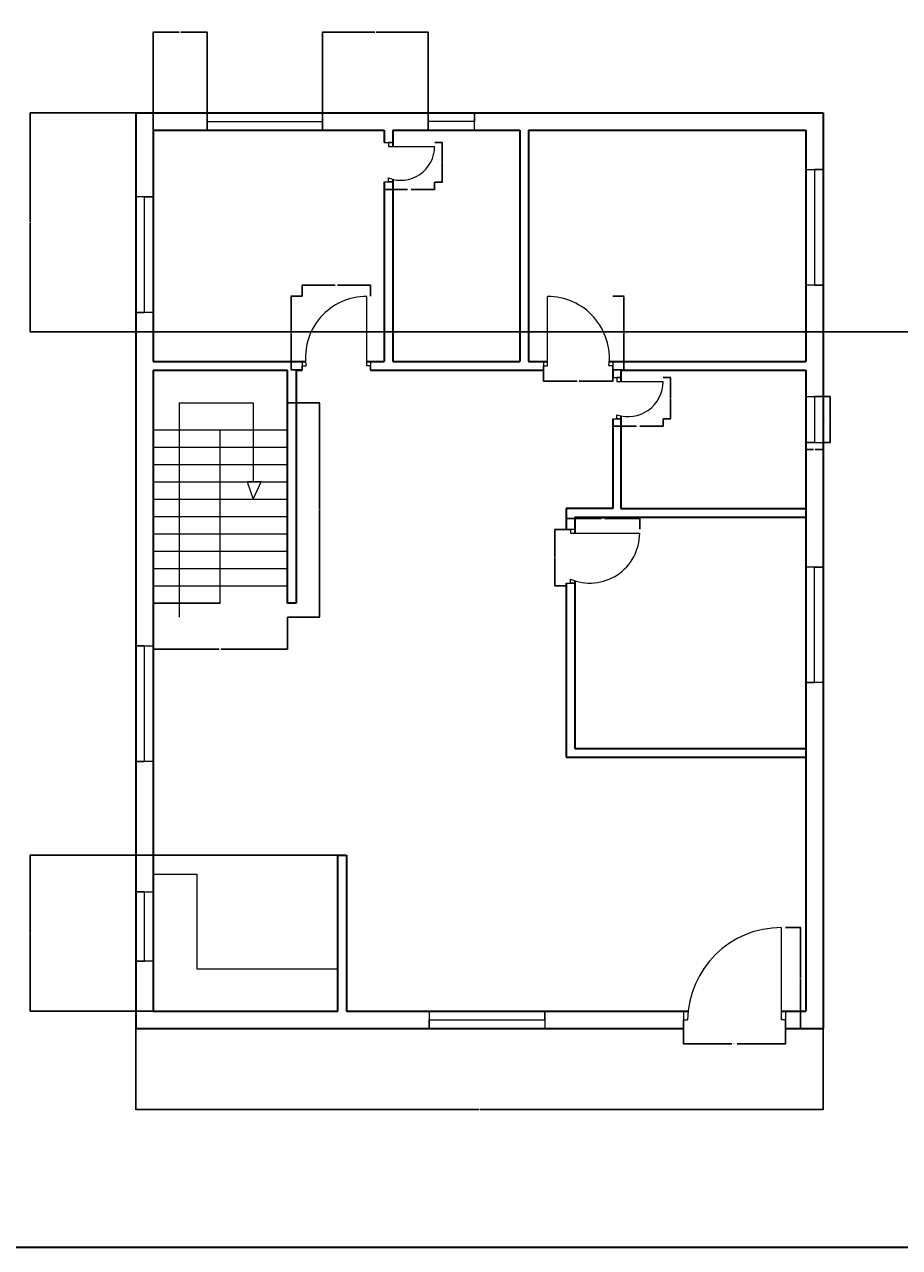
# Model space of a CAD drawing. Units: inches. Extents: x 1912 to 3731, y 1384 to 2459.
# Tile 6 of 8: x 2821 to 3276, y 1384 to 2019. Entities that reach past the tile are written whole.
import ezdxf

# ---------------------------------------------------------------- set-up
doc = ezdxf.new("R2010")
doc.units = ezdxf.units.IN
for name, color, linetype, lineweight in [('A-ANNO-DIMS', 2, 'Continuous', 18), ('A-ANNO-SYMB', 2, 'Continuous', 25), ('A-ANNO-TTLB', 7, 'Continuous', 35), ('A-DOOR', 3, 'Continuous', 20), ('A-FLOR-CASE', 8, 'Continuous', 20), ('A-FLOR-STRS', 7, 'Continuous', 18), ('A-GLAZ', 4, 'Continuous', 18), ('A-WALL', 7, 'Continuous', 35)]:
    doc.layers.add(name, color=color, linetype=linetype, lineweight=lineweight)
doc.styles.get("Standard").update_dxf_attribs({"font": 'arial.ttf'})
doc.dimstyles.get("Standard").update_dxf_attribs({"dimtxt": 0.18, "dimasz": 0.18, "dimexe": 0.18, "dimexo": 0.0625, "dimgap": 0.09, "dimtad": 0, "dimtih": 1, "dimtoh": 1, "dimdec": 4, "dimzin": 0, "dimdsep": 46, "dimtxsty": 'Standard', "dimcen": 0.09, "dimadec": 0, "dimazin": 0, "dimtfac": 1, "dimtdec": 4, "dimtofl": 0, "dimtmove": 0, "dimatfit": 3, "dimfxl": 1, "dimtolj": 1, "dimtzin": 0, "dimarcsym": 0})

# ---------------------------------------------------------------- blocks, each defined once
blk = doc.blocks.new('STAIR-RETURN-GROUND')
for p, q in [((13.73, 0), (13.73, 111.26)), ((13.73, 111.26), (52.04, 111.26)), ((52.04, 111.26), (52.04, 70.24)), ((0, 97.24), (34.87, 97.24)), ((34.87, 97.24), (69.75, 97.24)), ((34.87, 7.24), (34.87, 97.12)), ((0, 88.24), (34.87, 88.24)), ((34.87, 88.24), (69.75, 88.24)), ((0, 79.24), (34.87, 79.24)), ((34.87, 79.24), (69.75, 79.24)), ((0, 70.24), (34.87, 70.24)), ((34.87, 70.24), (69.75, 70.24)), ((56.12, 70.24), (48.82, 70.24)), ((48.82, 70.24), (52.04, 61.24)), ((52.04, 61.24), (56.12, 70.24)), ((0, 61.24), (34.87, 61.24)), ((34.87, 61.24), (69.75, 61.24)), ((0, 52.24), (34.87, 52.24)), ((34.87, 52.24), (69.75, 52.24)), ((0, 43.24), (34.87, 43.24)), ((34.87, 43.24), (69.75, 43.24)), ((0, 34.24), (34.87, 34.24)), ((34.87, 34.24), (69.75, 34.24)), ((0, 25.24), (34.87, 25.24)), ((34.87, 25.24), (69.75, 25.24)), ((0, 16.24), (34.87, 16.24)), ((34.87, 7.24), (34.87, 16.24)), ((34.87, 16.24), (69.75, 16.24)), ((34.87, 7.24), (0, 7.24)), ((0, 7.24), (34.87, 7.24))]:
    blk.add_line(p, q)
blk = doc.blocks.new('DOOR-36-GF-KIDS')
for p, q in [((2, 2.25), (2, 38.25)), ((0, 4.5), (0, 0)), ((0, 0), (0, 2.25)), ((0, 2.25), (2, 2.25)), ((35.93, 2.25), (33.93, 2.25)), ((35.93, 4.5), (35.93, 0)), ((35.93, 0), (35.93, 2.25))]:
    blk.add_line(p, q)
blk.add_arc((2, 6.09), 32.16, 353.14548, 90)
blk = doc.blocks.new('DOOR-36-GF-MASTER')
for p, q in [((33.51, 2.25), (33.51, 38.25)), ((0, 4.5), (0, 0)), ((0, 0), (0, 2.25)), ((0, 2.25), (2, 2.25)), ((35.51, 2.25), (33.51, 2.25)), ((35.51, 4.5), (35.51, 0)), ((35.51, 0), (35.51, 2.25))]:
    blk.add_line(p, q)
blk.add_arc((33.51, 6.46), 31.79, 90, 187.60289)
blk = doc.blocks.new('DOOR-24-GF-ENSUITE')
for p, q in [((0, 20.44), (4.5, 20.44)), ((4.5, 20.44), (2.25, 20.44)), ((2.25, 20.44), (2.25, 18.44)), ((2.25, 18.44), (26.25, 18.44)), ((2.25, 0), (2.25, 2)), ((0, 0), (4.5, 0)), ((4.5, 0), (2.25, 0))]:
    blk.add_line(p, q)
blk.add_arc((8.62, 18.44), 17.63, 248.8218, 0)
blk = doc.blocks.new('DOOR-24-GF-BATH')
for p, q in [((0, 21.32), (4.21, 21.32)), ((4.21, 21.32), (2.1, 21.32)), ((2.1, 21.32), (2.1, 19.32)), ((2.1, 19.32), (26.1, 19.32)), ((2.1, 0), (2.1, 2)), ((0, 0), (4.21, 0)), ((4.21, 0), (2.1, 0))]:
    blk.add_line(p, q)
blk.add_arc((7.86, 19.32), 18.25, 251.63069, 0)
blk = doc.blocks.new('DOOR-36-GF-FAMILY')
for p, q in [((4.5, 27.89), (0, 27.89)), ((0, 27.89), (2.25, 27.89)), ((2.25, 27.89), (2.25, 25.89)), ((2.25, 25.89), (38.25, 25.89)), ((0, 0.04), (4.5, 0.04)), ((2.25, 0.04), (2.25, 2.04)), ((4.5, 0.04), (2.25, 0.04))]:
    blk.add_line(p, q)
blk.add_arc((12.35, 25.89), 25.9, 247.04952, 0)
blk = doc.blocks.new('DOOR-48-ENTRY')
for p, q in [((50.83, 40.5), (50.83, 52.5)), ((50.83, 4.5), (50.83, 40.5)), ((0, 9), (0, 0)), ((52.83, 9), (52.83, 0)), ((0, 0), (0, 4.5)), ((0, 4.5), (2, 4.5)), ((52.83, 4.5), (50.83, 4.5)), ((52.83, 0), (52.83, 4.5))]:
    blk.add_line(p, q)
blk.add_arc((50.83, 3.66), 48.84, 90, 179.01371)
blk = doc.blocks.new('WIN-PLAN-60-A')
for p, q in [((0, 9), (0, 0)), ((60, 4.5), (60, 9)), ((60, 9), (60, 0)), ((0, 0), (0, 4.5)), ((0, 4.5), (60, 4.5))]:
    blk.add_line(p, q)
blk = doc.blocks.new('WIN-PLAN-60-B')
for p, q in [((0, 60), (9, 60)), ((9, 60), (4.5, 60)), ((4.5, 60), (4.5, 0)), ((9, 0), (0, 0)), ((4.5, 0), (9, 0))]:
    blk.add_line(p, q)
blk = doc.blocks.new('WIN-PLAN-24-A')
for p, q in [((0, 24), (9, 24)), ((9, 24), (4.5, 24)), ((4.5, 24), (4.5, 0)), ((4.5, 0), (0, 0)), ((0, 0), (9, 0))]:
    blk.add_line(p, q)
blk = doc.blocks.new('WIN-PLAN-36')
for p, q in [((4.5, 36), (0, 36)), ((0, 36), (9, 36)), ((4.5, 0), (4.5, 36)), ((9, 0), (0, 0)), ((0, 0), (4.5, 0))]:
    blk.add_line(p, q)
blk = doc.blocks.new('*D35')
at = {"layer": 'A-ANNO-DIMS', "color": 0, "lineweight": -2, "transparency": 16777216}
for p, q in [((3235.85, 1825.91), (3239.57, 1825.91)), ((3239.39, 1825.73), (3239.39, 1814.1)), ((3239.39, 1802.09), (3239.39, 1813.73)), ((3235.85, 1801.91), (3239.57, 1801.91))]:
    blk.add_line(p, q, dxfattribs=at)
at = {"layer": 'A-ANNO-DIMS', "color": 0, "transparency": 16777216}
for points in [[(3239.36, 1825.73), (3239.42, 1825.73), (3239.39, 1825.91)], [(3239.36, 1802.09), (3239.42, 1802.09), (3239.39, 1801.91)]]:
    blk.add_solid(points, dxfattribs=at)
at = {"layer": 'Defpoints', "color": 0, "transparency": 16777216}
for p in [(3235.79, 1825.91), (3239.39, 1825.91), (3235.79, 1801.91)]:
    blk.add_point(p, dxfattribs=at)
at = {"layer": 'A-ANNO-DIMS', "color": 0, "transparency": 16777216, "insert": (3239.39, 1813.91), "char_height": 0.18, "attachment_point": 5}
blk.add_mtext('\\A1;WC WINDOW 24 TYP.', dxfattribs=at)
blk = doc.blocks.new('*D36')
at = {"layer": 'A-ANNO-DIMS', "color": 0, "lineweight": -2, "transparency": 16777216}
for p, q in [((3226.79, 1801.85), (3226.79, 1798.13)), ((3226.97, 1798.31), (3230.83, 1798.31)), ((3235.61, 1798.31), (3231.74, 1798.31)), ((3235.79, 1801.85), (3235.79, 1798.13))]:
    blk.add_line(p, q, dxfattribs=at)
at = {"layer": 'A-ANNO-DIMS', "color": 0, "transparency": 16777216}
for points in [[(3226.97, 1798.34), (3226.97, 1798.28), (3226.79, 1798.31)], [(3235.61, 1798.34), (3235.61, 1798.28), (3235.79, 1798.31)]]:
    blk.add_solid(points, dxfattribs=at)
at = {"layer": 'Defpoints', "color": 0, "transparency": 16777216}
for p in [(3226.79, 1801.91), (3235.79, 1801.91), (3235.79, 1798.31)]:
    blk.add_point(p, dxfattribs=at)
at = {"layer": 'A-ANNO-DIMS', "color": 0, "transparency": 16777216, "insert": (3231.29, 1798.31), "char_height": 0.18, "attachment_point": 5}
blk.add_mtext('\\A1;9 TYP.', dxfattribs=at)
blk = doc.blocks.new('*D63')
at = {"layer": 'A-ANNO-DIMS', "color": 0, "lineweight": -2, "transparency": 16777216}
for p, q in [((2957.59, 1822.61), (2974.4, 1822.61)), ((2974.22, 1822.43), (2974.22, 1767.16)), ((2974.22, 1711.53), (2974.22, 1766.79)), ((2957.59, 1711.35), (2974.4, 1711.35))]:
    blk.add_line(p, q, dxfattribs=at)
at = {"layer": 'A-ANNO-DIMS', "color": 0, "transparency": 16777216}
for points in [[(2974.19, 1822.43), (2974.25, 1822.43), (2974.22, 1822.61)], [(2974.19, 1711.53), (2974.25, 1711.53), (2974.22, 1711.35)]]:
    blk.add_solid(points, dxfattribs=at)
at = {"layer": 'Defpoints', "color": 0, "transparency": 16777216}
for p in [(2957.53, 1822.61), (2974.22, 1822.61), (2957.53, 1711.35)]:
    blk.add_point(p, dxfattribs=at)
at = {"layer": 'A-ANNO-DIMS', "color": 0, "transparency": 16777216, "insert": (2974.22, 1766.98), "char_height": 0.18, "attachment_point": 5}
blk.add_mtext('\\A1;STAIR 111 TYP.', dxfattribs=at)
blk = doc.blocks.new('*D64')
at = {"layer": 'A-ANNO-DIMS', "color": 0, "lineweight": -2, "transparency": 16777216}
for p, q in [((2887.79, 1711.28), (2887.79, 1694.48)), ((2957.53, 1711.28), (2957.53, 1694.48)), ((2887.97, 1694.66), (2922.13, 1694.66)), ((2957.35, 1694.66), (2923.19, 1694.66))]:
    blk.add_line(p, q, dxfattribs=at)
at = {"layer": 'A-ANNO-DIMS', "color": 0, "transparency": 16777216}
for points in [[(2887.97, 1694.69), (2887.97, 1694.63), (2887.79, 1694.66)], [(2957.35, 1694.69), (2957.35, 1694.63), (2957.53, 1694.66)]]:
    blk.add_solid(points, dxfattribs=at)
at = {"layer": 'Defpoints', "color": 0, "transparency": 16777216}
for p in [(2887.79, 1711.35), (2957.53, 1711.35), (2957.53, 1694.66)]:
    blk.add_point(p, dxfattribs=at)
at = {"layer": 'A-ANNO-DIMS', "color": 0, "transparency": 16777216, "insert": (2922.66, 1694.66), "char_height": 0.18, "attachment_point": 5}
blk.add_mtext('\\A1;70 TYP.', dxfattribs=at)
blk = doc.blocks.new('*D67')
at = {"layer": 'A-ANNO-DIMS', "color": 0, "lineweight": -2, "transparency": 16777216}
for p, q in [((3126.64, 1877.88), (3132.49, 1877.88)), ((3132.31, 1877.7), (3132.31, 1858.93)), ((3132.31, 1839.81), (3132.31, 1858.57)), ((3126.64, 1839.63), (3132.49, 1839.63))]:
    blk.add_line(p, q, dxfattribs=at)
at = {"layer": 'A-ANNO-DIMS', "color": 0, "transparency": 16777216}
for points in [[(3132.28, 1877.7), (3132.34, 1877.7), (3132.31, 1877.88)], [(3132.28, 1839.81), (3132.34, 1839.81), (3132.31, 1839.63)]]:
    blk.add_solid(points, dxfattribs=at)
at = {"layer": 'Defpoints', "color": 0, "transparency": 16777216}
for p in [(3126.58, 1877.88), (3132.31, 1877.88), (3126.58, 1839.63)]:
    blk.add_point(p, dxfattribs=at)
at = {"layer": 'A-ANNO-DIMS', "color": 0, "transparency": 16777216, "insert": (3132.31, 1858.75), "char_height": 0.18, "attachment_point": 5}
blk.add_mtext('\\A1;DOOR 38 TYP.', dxfattribs=at)
blk = doc.blocks.new('*D68')
at = {"layer": 'A-ANNO-DIMS', "color": 0, "lineweight": -2, "transparency": 16777216}
for p, q in [((3090.64, 1839.56), (3090.64, 1833.71)), ((3126.58, 1839.56), (3126.58, 1833.71)), ((3090.82, 1833.89), (3108.08, 1833.89)), ((3126.4, 1833.89), (3109.14, 1833.89))]:
    blk.add_line(p, q, dxfattribs=at)
at = {"layer": 'A-ANNO-DIMS', "color": 0, "transparency": 16777216}
for points in [[(3090.82, 1833.92), (3090.82, 1833.86), (3090.64, 1833.89)], [(3126.4, 1833.92), (3126.4, 1833.86), (3126.58, 1833.89)]]:
    blk.add_solid(points, dxfattribs=at)
at = {"layer": 'Defpoints', "color": 0, "transparency": 16777216}
for p in [(3090.64, 1839.63), (3126.58, 1839.63), (3126.58, 1833.89)]:
    blk.add_point(p, dxfattribs=at)
at = {"layer": 'A-ANNO-DIMS', "color": 0, "transparency": 16777216, "insert": (3108.61, 1833.89), "char_height": 0.18, "attachment_point": 5}
blk.add_mtext('\\A1;36 TYP.', dxfattribs=at)
blk = doc.blocks.new('*D69')
at = {"layer": 'A-ANNO-DIMS', "color": 0, "lineweight": -2, "transparency": 16777216}
for p, q in [((2965.17, 1877.88), (2959.31, 1877.88)), ((2959.49, 1877.7), (2959.49, 1858.93)), ((2959.49, 1839.81), (2959.49, 1858.57)), ((2965.17, 1839.63), (2959.31, 1839.63))]:
    blk.add_line(p, q, dxfattribs=at)
at = {"layer": 'A-ANNO-DIMS', "color": 0, "transparency": 16777216}
for points in [[(2959.46, 1877.7), (2959.52, 1877.7), (2959.49, 1877.88)], [(2959.46, 1839.81), (2959.52, 1839.81), (2959.49, 1839.63)]]:
    blk.add_solid(points, dxfattribs=at)
at = {"layer": 'Defpoints', "color": 0, "transparency": 16777216}
for p in [(2959.49, 1877.88), (2965.23, 1877.88), (2965.23, 1839.63)]:
    blk.add_point(p, dxfattribs=at)
at = {"layer": 'A-ANNO-DIMS', "color": 0, "transparency": 16777216, "insert": (2959.49, 1858.75), "char_height": 0.18, "attachment_point": 5}
blk.add_mtext('\\A1;DOOR 38 TYP.', dxfattribs=at)
blk = doc.blocks.new('*D70')
at = {"layer": 'A-ANNO-DIMS', "color": 0, "lineweight": -2, "transparency": 16777216}
for p, q in [((2965.23, 1877.94), (2965.23, 1883.79)), ((2965.41, 1883.61), (2982.46, 1883.61)), ((3000.56, 1883.61), (2983.51, 1883.61)), ((3000.74, 1877.94), (3000.74, 1883.79))]:
    blk.add_line(p, q, dxfattribs=at)
at = {"layer": 'A-ANNO-DIMS', "color": 0, "transparency": 16777216}
for points in [[(2965.41, 1883.64), (2965.41, 1883.58), (2965.23, 1883.61)], [(3000.56, 1883.64), (3000.56, 1883.58), (3000.74, 1883.61)]]:
    blk.add_solid(points, dxfattribs=at)
at = {"layer": 'Defpoints', "color": 0, "transparency": 16777216}
for p in [(3000.74, 1883.61), (2965.23, 1877.88), (3000.74, 1877.88)]:
    blk.add_point(p, dxfattribs=at)
at = {"layer": 'A-ANNO-DIMS', "color": 0, "transparency": 16777216, "insert": (2982.99, 1883.61), "char_height": 0.18, "attachment_point": 5}
blk.add_mtext('\\A1;36 TYP.', dxfattribs=at)
blk = doc.blocks.new('*D71')
at = {"layer": 'A-ANNO-DIMS', "color": 0, "lineweight": -2, "transparency": 16777216}
for p, q in [((3007.79, 1937.16), (3007.79, 1933.11)), ((3034.04, 1937.16), (3034.04, 1933.11)), ((3007.97, 1933.29), (3019.97, 1933.29)), ((3033.86, 1933.29), (3021.85, 1933.29))]:
    blk.add_line(p, q, dxfattribs=at)
at = {"layer": 'A-ANNO-DIMS', "color": 0, "transparency": 16777216}
for points in [[(3007.97, 1933.32), (3007.97, 1933.26), (3007.79, 1933.29)], [(3033.86, 1933.32), (3033.86, 1933.26), (3034.04, 1933.29)]]:
    blk.add_solid(points, dxfattribs=at)
at = {"layer": 'Defpoints', "color": 0, "transparency": 16777216}
for p in [(3007.79, 1937.22), (3034.04, 1937.22), (3034.04, 1933.29)]:
    blk.add_point(p, dxfattribs=at)
at = {"layer": 'A-ANNO-DIMS', "color": 0, "transparency": 16777216, "insert": (3020.91, 1933.29), "char_height": 0.18, "attachment_point": 5}
blk.add_mtext('\\A1;DOOR 26 TYP.', dxfattribs=at)
blk = doc.blocks.new('*D72')
at = {"layer": 'A-ANNO-DIMS', "color": 0, "lineweight": -2, "transparency": 16777216}
for p, q in [((3034.1, 1957.76), (3038.15, 1957.76)), ((3037.97, 1957.58), (3037.97, 1947.67)), ((3037.97, 1937.4), (3037.97, 1947.31)), ((3034.1, 1937.22), (3038.15, 1937.22))]:
    blk.add_line(p, q, dxfattribs=at)
at = {"layer": 'A-ANNO-DIMS', "color": 0, "transparency": 16777216}
for points in [[(3037.94, 1957.58), (3038, 1957.58), (3037.97, 1957.76)], [(3037.94, 1937.4), (3038, 1937.4), (3037.97, 1937.22)]]:
    blk.add_solid(points, dxfattribs=at)
at = {"layer": 'Defpoints', "color": 0, "transparency": 16777216}
for p in [(3034.04, 1957.76), (3037.97, 1957.76), (3034.04, 1937.22)]:
    blk.add_point(p, dxfattribs=at)
at = {"layer": 'A-ANNO-DIMS', "color": 0, "transparency": 16777216, "insert": (3037.97, 1947.49), "char_height": 0.18, "attachment_point": 5}
blk.add_mtext('\\A1;21 TYP.', dxfattribs=at)
blk = doc.blocks.new('*D73')
at = {"layer": 'A-ANNO-DIMS', "color": 0, "lineweight": -2, "transparency": 16777216}
for p, q in [((3126.58, 1814.27), (3126.58, 1810.23)), ((3126.76, 1810.41), (3138.69, 1810.41)), ((3152.5, 1810.41), (3140.56, 1810.41)), ((3152.68, 1814.27), (3152.68, 1810.23))]:
    blk.add_line(p, q, dxfattribs=at)
at = {"layer": 'A-ANNO-DIMS', "color": 0, "transparency": 16777216}
for points in [[(3126.76, 1810.44), (3126.76, 1810.38), (3126.58, 1810.41)], [(3152.5, 1810.44), (3152.5, 1810.38), (3152.68, 1810.41)]]:
    blk.add_solid(points, dxfattribs=at)
at = {"layer": 'Defpoints', "color": 0, "transparency": 16777216}
for p in [(3126.58, 1814.33), (3152.68, 1814.33), (3152.68, 1810.41)]:
    blk.add_point(p, dxfattribs=at)
at = {"layer": 'A-ANNO-DIMS', "color": 0, "transparency": 16777216, "insert": (3139.63, 1810.41), "char_height": 0.18, "attachment_point": 5}
blk.add_mtext('\\A1;DOOR 26 TYP.', dxfattribs=at)
blk = doc.blocks.new('*D74')
at = {"layer": 'A-ANNO-DIMS', "color": 0, "lineweight": -2, "transparency": 16777216}
for p, q in [((3152.74, 1835.65), (3156.78, 1835.65)), ((3156.6, 1835.47), (3156.6, 1825.17)), ((3156.6, 1814.51), (3156.6, 1824.81)), ((3152.74, 1814.33), (3156.78, 1814.33))]:
    blk.add_line(p, q, dxfattribs=at)
at = {"layer": 'A-ANNO-DIMS', "color": 0, "transparency": 16777216}
for points in [[(3156.57, 1835.47), (3156.63, 1835.47), (3156.6, 1835.65)], [(3156.57, 1814.51), (3156.63, 1814.51), (3156.6, 1814.33)]]:
    blk.add_solid(points, dxfattribs=at)
at = {"layer": 'Defpoints', "color": 0, "transparency": 16777216}
for p in [(3152.68, 1835.65), (3156.6, 1835.65), (3152.68, 1814.33)]:
    blk.add_point(p, dxfattribs=at)
at = {"layer": 'A-ANNO-DIMS', "color": 0, "transparency": 16777216, "insert": (3156.6, 1824.99), "char_height": 0.18, "attachment_point": 5}
blk.add_mtext('\\A1;21 TYP.', dxfattribs=at)
blk = doc.blocks.new('*D75')
at = {"layer": 'A-ANNO-DIMS', "color": 0, "lineweight": -2, "transparency": 16777216}
for p, q in [((3102.29, 1756.92), (3102.29, 1762.78)), ((3102.47, 1762.6), (3120.47, 1762.6)), ((3140.36, 1762.6), (3122.35, 1762.6)), ((3140.54, 1756.92), (3140.54, 1762.78))]:
    blk.add_line(p, q, dxfattribs=at)
at = {"layer": 'A-ANNO-DIMS', "color": 0, "transparency": 16777216}
for points in [[(3102.47, 1762.63), (3102.47, 1762.57), (3102.29, 1762.6)], [(3140.36, 1762.63), (3140.36, 1762.57), (3140.54, 1762.6)]]:
    blk.add_solid(points, dxfattribs=at)
at = {"layer": 'Defpoints', "color": 0, "transparency": 16777216}
for p in [(3140.54, 1762.6), (3102.29, 1756.86), (3140.54, 1756.86)]:
    blk.add_point(p, dxfattribs=at)
at = {"layer": 'A-ANNO-DIMS', "color": 0, "transparency": 16777216, "insert": (3121.41, 1762.6), "char_height": 0.18, "attachment_point": 5}
blk.add_mtext('\\A1;DOOR 38 TYP.', dxfattribs=at)
blk = doc.blocks.new('*D76')
at = {"layer": 'A-ANNO-DIMS', "color": 0, "lineweight": -2, "transparency": 16777216}
for p, q in [((3102.22, 1756.86), (3096.37, 1756.86)), ((3096.55, 1756.68), (3096.55, 1742.42)), ((3096.55, 1727.8), (3096.55, 1742.06)), ((3102.22, 1727.62), (3096.37, 1727.62))]:
    blk.add_line(p, q, dxfattribs=at)
at = {"layer": 'A-ANNO-DIMS', "color": 0, "transparency": 16777216}
for points in [[(3096.52, 1756.68), (3096.58, 1756.68), (3096.55, 1756.86)], [(3096.52, 1727.8), (3096.58, 1727.8), (3096.55, 1727.62)]]:
    blk.add_solid(points, dxfattribs=at)
at = {"layer": 'Defpoints', "color": 0, "transparency": 16777216}
for p in [(3096.55, 1756.86), (3102.29, 1756.86), (3102.29, 1727.62)]:
    blk.add_point(p, dxfattribs=at)
at = {"layer": 'A-ANNO-DIMS', "color": 0, "transparency": 16777216, "insert": (3096.55, 1742.24), "char_height": 0.18, "attachment_point": 5}
blk.add_mtext('\\A1;29 TYP.', dxfattribs=at)
blk = doc.blocks.new('*D77')
at = {"layer": 'A-ANNO-DIMS', "color": 0, "lineweight": -2, "transparency": 16777216}
for p, q in [((3163.37, 1497.56), (3163.37, 1489.52)), ((3216.21, 1497.56), (3216.21, 1489.52)), ((3163.55, 1489.7), (3188.39, 1489.7)), ((3216.03, 1489.7), (3191.19, 1489.7))]:
    blk.add_line(p, q, dxfattribs=at)
at = {"layer": 'A-ANNO-DIMS', "color": 0, "transparency": 16777216}
for points in [[(3163.55, 1489.73), (3163.55, 1489.67), (3163.37, 1489.7)], [(3216.03, 1489.73), (3216.03, 1489.67), (3216.21, 1489.7)]]:
    blk.add_solid(points, dxfattribs=at)
at = {"layer": 'Defpoints', "color": 0, "transparency": 16777216}
for p in [(3163.37, 1497.63), (3216.21, 1497.63), (3216.21, 1489.7)]:
    blk.add_point(p, dxfattribs=at)
at = {"layer": 'A-ANNO-DIMS', "color": 0, "transparency": 16777216, "insert": (3189.79, 1489.7), "char_height": 0.18, "attachment_point": 5}
blk.add_mtext('\\A1;ENTRY DOOR 53 TYP.', dxfattribs=at)
blk = doc.blocks.new('*D78')
at = {"layer": 'A-ANNO-DIMS', "color": 0, "lineweight": -2, "transparency": 16777216}
for p, q in [((3216.27, 1550.13), (3224.31, 1550.13)), ((3224.13, 1549.95), (3224.13, 1524.06)), ((3224.13, 1497.81), (3224.13, 1523.69)), ((3216.27, 1497.63), (3224.31, 1497.63))]:
    blk.add_line(p, q, dxfattribs=at)
at = {"layer": 'A-ANNO-DIMS', "color": 0, "transparency": 16777216}
for points in [[(3224.1, 1549.95), (3224.16, 1549.95), (3224.13, 1550.13)], [(3224.1, 1497.81), (3224.16, 1497.81), (3224.13, 1497.63)]]:
    blk.add_solid(points, dxfattribs=at)
at = {"layer": 'Defpoints', "color": 0, "transparency": 16777216}
for p in [(3216.21, 1550.13), (3224.13, 1550.13), (3216.21, 1497.63)]:
    blk.add_point(p, dxfattribs=at)
at = {"layer": 'A-ANNO-DIMS', "color": 0, "transparency": 16777216, "insert": (3224.13, 1523.88), "char_height": 0.18, "attachment_point": 5}
blk.add_mtext('\\A1;53 TYP.', dxfattribs=at)
blk = doc.blocks.new('*D105')
at = {"layer": 'A-ANNO-DIMS', "color": 0, "lineweight": -2, "transparency": 16777216}
for p, q in [((2878.79, 1497.56), (2878.79, 1455.5)), ((3235.79, 1497.56), (3235.79, 1455.5)), ((2878.97, 1455.68), (3057, 1455.68)), ((3235.61, 1455.68), (3057.57, 1455.68))]:
    blk.add_line(p, q, dxfattribs=at)
at = {"layer": 'A-ANNO-DIMS', "color": 0, "transparency": 16777216}
for points in [[(2878.97, 1455.71), (2878.97, 1455.65), (2878.79, 1455.68)], [(3235.61, 1455.71), (3235.61, 1455.65), (3235.79, 1455.68)]]:
    blk.add_solid(points, dxfattribs=at)
at = {"layer": 'Defpoints', "color": 0, "transparency": 16777216}
for p in [(2878.79, 1497.63), (3235.79, 1497.63), (3235.79, 1455.68)]:
    blk.add_point(p, dxfattribs=at)
at = {"layer": 'A-ANNO-DIMS', "color": 0, "transparency": 16777216, "insert": (3057.29, 1455.68), "char_height": 0.18, "attachment_point": 5}
blk.add_mtext('\\A1;357', dxfattribs=at)
blk = doc.blocks.new('*D108')
at = {"layer": 'A-ANNO-DIMS', "color": 0, "lineweight": -2, "transparency": 16777216}
for p, q in [((2878.72, 1973.13), (2823.71, 1973.13)), ((2823.89, 1972.95), (2823.89, 1916.48)), ((2823.89, 1859.65), (2823.89, 1916.11)), ((2865.78, 1859.47), (2823.71, 1859.47))]:
    blk.add_line(p, q, dxfattribs=at)
at = {"layer": 'A-ANNO-DIMS', "color": 0, "transparency": 16777216}
for points in [[(2823.86, 1972.95), (2823.92, 1972.95), (2823.89, 1973.13)], [(2823.86, 1859.65), (2823.92, 1859.65), (2823.89, 1859.47)]]:
    blk.add_solid(points, dxfattribs=at)
at = {"layer": 'Defpoints', "color": 0, "transparency": 16777216}
for p in [(2878.79, 1973.13), (2823.89, 1859.47), (2865.84, 1859.47)]:
    blk.add_point(p, dxfattribs=at)
at = {"layer": 'A-ANNO-DIMS', "color": 0, "transparency": 16777216, "insert": (2823.89, 1916.3), "char_height": 0.18, "attachment_point": 5}
blk.add_mtext('\\A1;113.66', dxfattribs=at)
blk = doc.blocks.new('*D109')
at = {"layer": 'A-ANNO-DIMS', "color": 0, "lineweight": -2, "transparency": 16777216}
for p, q in [((2887.79, 1964.19), (2887.79, 2015.26)), ((2887.97, 2015.08), (2901.41, 2015.08)), ((2915.64, 2015.08), (2902.2, 2015.08)), ((2915.82, 1964.19), (2915.82, 2015.26))]:
    blk.add_line(p, q, dxfattribs=at)
at = {"layer": 'A-ANNO-DIMS', "color": 0, "transparency": 16777216}
for points in [[(2887.97, 2015.11), (2887.97, 2015.05), (2887.79, 2015.08)], [(2915.64, 2015.11), (2915.64, 2015.05), (2915.82, 2015.08)]]:
    blk.add_solid(points, dxfattribs=at)
at = {"layer": 'Defpoints', "color": 0, "transparency": 16777216}
for p in [(2915.82, 2015.08), (2887.79, 1964.13), (2915.82, 1964.13)]:
    blk.add_point(p, dxfattribs=at)
at = {"layer": 'A-ANNO-DIMS', "color": 0, "transparency": 16777216, "insert": (2901.8, 2015.08), "char_height": 0.18, "attachment_point": 5}
blk.add_mtext('\\A1;28.03', dxfattribs=at)
blk = doc.blocks.new('*D110')
at = {"layer": 'A-ANNO-DIMS', "color": 0, "lineweight": -2, "transparency": 16777216}
for p, q in [((2975.82, 1964.19), (2975.82, 2015.26)), ((2976, 2015.08), (3002.89, 2015.08)), ((3030.56, 2015.08), (3003.67, 2015.08)), ((3030.74, 1964.19), (3030.74, 2015.26))]:
    blk.add_line(p, q, dxfattribs=at)
at = {"layer": 'A-ANNO-DIMS', "color": 0, "transparency": 16777216}
for points in [[(2976, 2015.11), (2976, 2015.05), (2975.82, 2015.08)], [(3030.56, 2015.11), (3030.56, 2015.05), (3030.74, 2015.08)]]:
    blk.add_solid(points, dxfattribs=at)
at = {"layer": 'Defpoints', "color": 0, "transparency": 16777216}
for p in [(3030.74, 2015.08), (2975.82, 1964.13), (3030.74, 1964.13)]:
    blk.add_point(p, dxfattribs=at)
at = {"layer": 'A-ANNO-DIMS', "color": 0, "transparency": 16777216, "insert": (3003.28, 2015.08), "char_height": 0.18, "attachment_point": 5}
blk.add_mtext('\\A1;54.92', dxfattribs=at)
blk = doc.blocks.new('*D111')
at = {"layer": 'A-ANNO-DIMS', "color": 0, "lineweight": -2, "transparency": 16777216}
for p, q in [((2983.72, 1587.72), (2823.71, 1587.72)), ((2823.89, 1587.54), (2823.89, 1547.35)), ((2823.89, 1506.81), (2823.89, 1546.99)), ((2983.72, 1506.63), (2823.71, 1506.63))]:
    blk.add_line(p, q, dxfattribs=at)
at = {"layer": 'A-ANNO-DIMS', "color": 0, "transparency": 16777216}
for points in [[(2823.86, 1587.54), (2823.92, 1587.54), (2823.89, 1587.72)], [(2823.86, 1506.81), (2823.92, 1506.81), (2823.89, 1506.63)]]:
    blk.add_solid(points, dxfattribs=at)
at = {"layer": 'Defpoints', "color": 0, "transparency": 16777216}
for p in [(2823.89, 1587.72), (2983.79, 1587.72), (2983.79, 1506.63)]:
    blk.add_point(p, dxfattribs=at)
at = {"layer": 'A-ANNO-DIMS', "color": 0, "transparency": 16777216, "insert": (2823.89, 1547.17), "char_height": 0.18, "attachment_point": 5}
blk.add_mtext('\\A1;81.09', dxfattribs=at)

msp = doc.modelspace()

# ---------------------------------------------------------------- linework, layer by layer
at = {"layer": 'A-ANNO-SYMB'}
msp.add_line((2865.8394, 1859.4655), (3689.1639, 1859.4655), dxfattribs=at)
at = {"layer": 'A-ANNO-TTLB'}
msp.add_lwpolyline([(1912.2029, 2458.5537), (3720.218, 2458.5537), (3720.218, 1383.9599), (1912.2029, 1383.9599)], close=True, dxfattribs=at)
at = {"layer": 'A-FLOR-CASE'}
for p, q in [((2887.7856, 1577.7784), (2910.5279, 1577.7784)), ((2910.5279, 1577.7784), (2910.5279, 1528.7615)), ((2910.5279, 1528.7615), (2983.7856, 1528.7615))]:
    msp.add_line(p, q, dxfattribs=at)
at = {"layer": 'A-WALL'}
for p, q in [((2878.7856, 1973.1258), (2878.7856, 1497.6258)), ((2878.7856, 1973.1258), (2878.7856, 1497.6258)), ((2878.7856, 1973.1258), (3235.7856, 1973.1258)), ((3235.7856, 1973.1258), (3235.7856, 1497.6258)), ((2887.7856, 1964.1258), (2887.7856, 1844.1258)), ((2887.7856, 1964.1258), (3007.7856, 1964.1258)), ((3007.7856, 1964.1258), (3007.7856, 1957.7644)), ((3012.2856, 1964.1258), (3012.2856, 1955.7644)), ((3012.2856, 1964.1258), (3078.2856, 1964.1258)), ((3078.2856, 1964.1258), (3078.2856, 1844.1258)), ((3082.7856, 1964.1258), (3082.7856, 1844.1258)), ((3082.7856, 1964.1258), (3226.7856, 1964.1258)), ((3226.7856, 1964.1258), (3226.7856, 1844.1258)), ((3007.7856, 1937.3245), (3007.7856, 1844.1258)), ((3012.2856, 1938.6218), (3012.2856, 1844.1258)), ((2887.7856, 1844.1258), (2967.0091, 1844.1258)), ((2998.7424, 1844.1258), (3007.7856, 1844.1258)), ((3012.2856, 1844.1258), (3078.2856, 1844.1258)), ((3082.7856, 1844.1258), (3092.644, 1844.1258)), ((3124.7663, 1844.1258), (3226.7856, 1844.1258)), ((2887.7856, 1839.6258), (2887.7856, 1506.6258)), ((2887.7856, 1839.6258), (2957.5322, 1839.6258)), ((2957.5322, 1718.5838), (2957.5322, 1839.6258)), ((2962.0322, 1839.6258), (2965.2283, 1839.6258)), ((2962.0322, 1839.6258), (2962.0322, 1718.5838)), ((3000.7424, 1839.6258), (3090.644, 1839.6258)), ((3126.5756, 1839.6258), (3126.5756, 1835.6488)), ((3130.7856, 1839.6258), (3130.7856, 1833.6488)), ((3130.7856, 1839.6258), (3226.7856, 1839.6258)), ((3226.7856, 1839.6258), (3226.7856, 1506.6258)), ((3126.5756, 1814.3297), (3126.5756, 1767.6258)), ((3130.7856, 1815.7678), (3130.7856, 1767.6258)), ((3102.2856, 1767.6258), (3102.2856, 1756.8604)), ((3126.5756, 1767.6258), (3102.2856, 1767.6258)), ((3102.2856, 1767.6258), (3102.2856, 1763.1258)), ((3130.7856, 1767.6258), (3226.7856, 1767.6258)), ((3106.7856, 1763.1258), (3106.7856, 1754.8604)), ((3106.7856, 1763.1258), (3126.5756, 1763.1258)), ((3126.5756, 1763.1258), (3226.7856, 1763.1258)), ((3102.2856, 1729.0101), (3102.2856, 1638.6258)), ((3106.7856, 1730.178), (3106.7856, 1643.1258)), ((2962.0322, 1718.5838), (2957.5322, 1718.5838)), ((3102.2856, 1638.6258), (3226.7856, 1638.6258)), ((3106.7856, 1643.1258), (3226.7856, 1643.1258)), ((2983.7856, 1506.6258), (2983.7856, 1587.7153)), ((2983.7856, 1587.7153), (2988.2856, 1587.7153)), ((2988.2856, 1587.7153), (2988.2856, 1506.6258)), ((2887.7856, 1506.6258), (2983.7856, 1506.6258)), ((2887.7856, 1506.6258), (2983.7856, 1506.6258)), ((2988.2856, 1506.6258), (3165.659, 1506.6258)), ((3214.2068, 1506.6258), (3226.7856, 1506.6258)), ((2878.7856, 1497.6258), (3163.3733, 1497.6258)), ((3216.2068, 1497.6258), (3235.7856, 1497.6258))]:
    msp.add_line(p, q, dxfattribs=at)

# ---------------------------------------------------------------- block references
at = {"layer": 'A-DOOR'}
for name, p in [('DOOR-24-GF-ENSUITE', (3007.7858, 1937.325)), ('DOOR-36-GF-MASTER', (2965.2278, 1839.626)), ('DOOR-36-GF-KIDS', (3090.6438, 1839.626)), ('DOOR-24-GF-BATH', (3126.5758, 1814.33)), ('DOOR-36-GF-FAMILY', (3102.2858, 1728.971)), ('DOOR-48-ENTRY', (3163.3728, 1497.626))]:
    msp.add_blockref(name, p, dxfattribs=at)
at = {"layer": 'A-FLOR-STRS'}
msp.add_blockref('STAIR-RETURN-GROUND', (2887.7858, 1711.346), dxfattribs=at)
at = {"layer": 'A-GLAZ'}
for name, p in [('WIN-PLAN-60-A', (2915.8176, 1964.126)), ('WIN-PLAN-60-B', (3226.7858, 1883.676)), ('WIN-PLAN-24-A', (3226.7858, 1801.913)), ('WIN-PLAN-36', (2878.7858, 1532.687)), ('WIN-PLAN-60-A', (3031.2578, 1497.626))]:
    msp.add_blockref(name, p, dxfattribs=at)
at = {"layer": 'A-GLAZ', "extrusion": (0, 0, -1), "zscale": -1, "rotation": 90}
for name, p in [('WIN-PLAN-24-A', (-3030.7425, 1964.126)), ('WIN-PLAN-60-A', (-2878.7859, 1869.4675)), ('WIN-PLAN-60-A', (-3226.7859, 1677.3214))]:
    msp.add_blockref(name, p, dxfattribs=at)
at = {"layer": 'A-GLAZ', "rotation": 180}
msp.add_blockref('WIN-PLAN-60-B', (2887.7854, 1696.3403), dxfattribs=at)

# ---------------------------------------------------------------- dimensions: what is measured, and where the dimension line sits
at = {"layer": 'A-ANNO-DIMS'}
for base, p1, p2, override, picture, middle in [((2915.8175, 2015.0758), (2887.7856, 1964.1258), (2915.8175, 1964.1258), {"dimdec": 2, "dimlfac": 1, "dimrnd": 0, "dimzin": 0, "dimdsep": 46, "dimlunit": 2}, '*D109', (2901.8016, 2015.0758)), ((3030.742, 2015.0758), (2975.8175, 1964.1258), (3030.742, 1964.1258), {"dimdec": 2, "dimlfac": 1, "dimrnd": 0, "dimzin": 0, "dimdsep": 46, "dimlunit": 2}, '*D110', (3003.2798, 2015.0758)), ((3235.7856, 1455.6758), (2878.7856, 1497.6258), (3235.7856, 1497.6258), {"dimdec": 0, "dimlfac": 1, "dimrnd": 0, "dimzin": 0, "dimdsep": 46, "dimlunit": 2}, '*D105', (3057.2856, 1455.6758))]:
    dim = msp.add_linear_dim(base=base, p1=p1, p2=p2, dimstyle='Standard', override=override, dxfattribs=at)
    dim.commit()
    dim.dimension.update_dxf_attribs({"geometry": picture, "text_midpoint": middle})
for base, p1, p2, picture, middle in [((2823.8894, 1859.4655), (2878.7856, 1973.1258), (2865.8394, 1859.4655), '*D108', (2823.8894, 1916.2956)), ((2823.8894, 1587.7153), (2983.7856, 1506.6258), (2983.7856, 1587.7153), '*D111', (2823.8894, 1547.1705))]:
    dim = msp.add_linear_dim(base=base, p1=p1, p2=p2, angle=90, dimstyle='Standard', override={"dimdec": 2, "dimlfac": 1, "dimrnd": 0, "dimzin": 0, "dimdsep": 46, "dimlunit": 2}, dxfattribs=at)
    dim.commit()
    dim.dimension.update_dxf_attribs({"geometry": picture, "text_midpoint": middle})
for base, p1, p2, text, picture, middle in [((3037.9731, 1957.7644), (3034.0356, 1937.2233), (3034.0356, 1957.7644), '<> TYP.', '*D72', (3037.9731, 1947.4938)), ((2959.4908, 1877.8758), (2965.2283, 1839.6258), (2965.2283, 1877.8758), 'DOOR <> TYP.', '*D69', (2959.4908, 1858.7508)), ((3132.3131, 1877.8758), (3126.5756, 1839.6258), (3126.5756, 1877.8758), 'DOOR <> TYP.', '*D67', (3132.3131, 1858.7508)), ((3156.5964, 1835.6488), (3152.6806, 1814.3297), (3152.6806, 1835.6488), '<> TYP.', '*D74', (3156.5964, 1824.9893)), ((3239.3856, 1825.9126), (3235.7856, 1801.9126), (3235.7856, 1825.9126), 'WC WINDOW <> TYP.', '*D35', (3239.3856, 1813.9126)), ((2974.221, 1822.605), (2957.5322, 1711.3457), (2957.5322, 1822.605), 'STAIR <> TYP.', '*D63', (2974.221, 1766.9754)), ((3096.5481, 1756.8604), (3102.2856, 1727.623), (3102.2856, 1756.8604), '<> TYP.', '*D76', (3096.5481, 1742.2417)), ((3224.1318126599, 1550.1257615483), (3216.2067926195, 1497.6257615483), (3216.2067926195, 1550.1257615483), '<> TYP.', '*D78', (3224.1318126599, 1523.8757615483))]:
    dim = msp.add_linear_dim(base=base, p1=p1, p2=p2, angle=90, text=text, dimstyle='Standard', override={"dimdec": 0, "dimlfac": 1, "dimrnd": 0, "dimzin": 0, "dimdsep": 46, "dimlunit": 2}, dxfattribs=at)
    dim.commit()
    dim.dimension.update_dxf_attribs({"geometry": picture, "text_midpoint": middle})
for base, p1, p2, text, picture, middle in [((3034.0356, 1933.2858), (3007.7856, 1937.2233), (3034.0356, 1937.2233), 'DOOR <> TYP.', '*D71', (3020.9106, 1933.2858)), ((3000.7424, 1883.6133), (2965.2283, 1877.8758), (3000.7424, 1877.8758), '<> TYP.', '*D70', (2982.9853, 1883.6133)), ((3126.5756, 1833.8883), (3090.644, 1839.6258), (3126.5756, 1839.6258), '<> TYP.', '*D68', (3108.6098, 1833.8883)), ((3152.6806, 1810.414), (3126.5756, 1814.3297), (3152.6806, 1814.3297), 'DOOR <> TYP.', '*D73', (3139.6281, 1810.414)), ((3235.7856, 1798.3126), (3226.7856, 1801.9126), (3235.7856, 1801.9126), '<> TYP.', '*D36', (3231.2856, 1798.3126)), ((3140.5356, 1762.5979), (3102.2856, 1756.8604), (3140.5356, 1756.8604), 'DOOR <> TYP.', '*D75', (3121.4106, 1762.5979)), ((2957.5322, 1694.6568), (2887.7856, 1711.3457), (2957.5322, 1711.3457), '<> TYP.', '*D64', (2922.6589, 1694.6568)), ((3216.2068, 1489.7007), (3163.3733, 1497.6258), (3216.2068, 1497.6258), 'ENTRY DOOR <> TYP.', '*D77', (3189.7901, 1489.7007))]:
    dim = msp.add_linear_dim(base=base, p1=p1, p2=p2, text=text, dimstyle='Standard', override={"dimdec": 0, "dimlfac": 1, "dimrnd": 0, "dimzin": 0, "dimdsep": 46, "dimlunit": 2}, dxfattribs=at)
    dim.commit()
    dim.dimension.update_dxf_attribs({"geometry": picture, "text_midpoint": middle})

doc.saveas('drawing.dxf')
